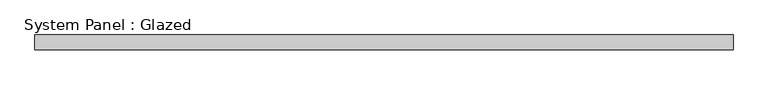
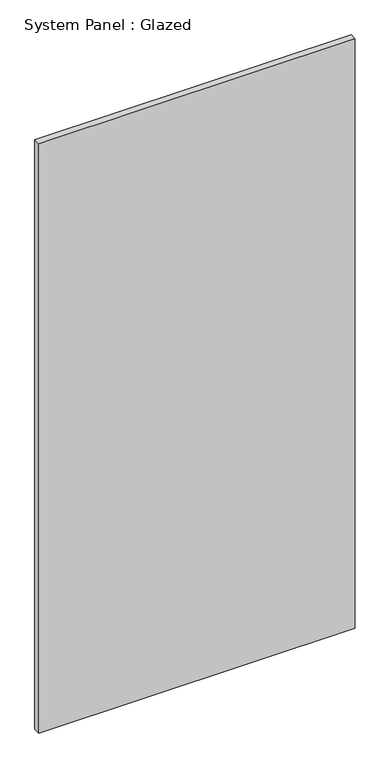
"""IFC4 building model written with IfcOpenShell, lengths in millimetres: plate geometry, System Panel : Glazed."""

from ifc_helpers import new_model, si_unit, origin, origin_with_axes, place, context, project, spatial, polyline, outline, extrude, source, transform, mapped, element, save


def system_panel_glazed_8a2d2adf(model_context):
    return source(origin(), model_context, "Body", "SweptSolid", [
        extrude(outline(polyline([(595.3125, 19.05), (-595.3125, 19.05), (-595.3125, 44.45), (595.3125, 44.45), (595.3125, 19.05)])), origin_with_axes(), (0.0, 0.0, 1.0), 2343.15),
    ])


if __name__ == "__main__":
    model = new_model("IFC4")
    model_context = context("Model", 3, world=origin())
    ifc_project = project(units=[si_unit("LENGTHUNIT", "METRE", prefix="MILLI")], contexts=[model_context])
    site = spatial("IfcSite", under=ifc_project)
    building = spatial("IfcBuilding", under=site)
    placement = place(None, origin())
    system_panel_glazed_shape = system_panel_glazed_8a2d2adf(model_context)
    element("IfcPlate", 1, ObjectType="System Panel : Glazed", at=placement, inside=building, context=model_context, shape_type="MappedRepresentation", body=[
        mapped(system_panel_glazed_shape, transform((0.0, 0.0, 0.0), x_axis=(1.0, 0.0, 0.0), y_axis=(0.0, 1.0, 0.0), z_axis=(0.0, 0.0, 1.0))),
    ])
    save(model, "model.ifc")

# Revit data of these elements
# Type "System Panel : Glazed"
#   Construction Type Id = "GSP4R"
#   Analytic Construction = "1/8 in Pilkington single glazing"
#   Visual Light Transmittance = 0.9
#   Solar Heat Gain Coefficient = 0.86
#   Heat Transfer Coefficient (U) = 1.18115 BTU/(h·ft²·°F)
# Element 1 (IfcPlate, "System Panel : Glazed")
#   Materials on its faces: "Glass"
# Materials
#   "Glass": class "Glass", colour RGB 0 128 192, transparency 0.75, Description = "Soda Lime Glass", Cost = 0
